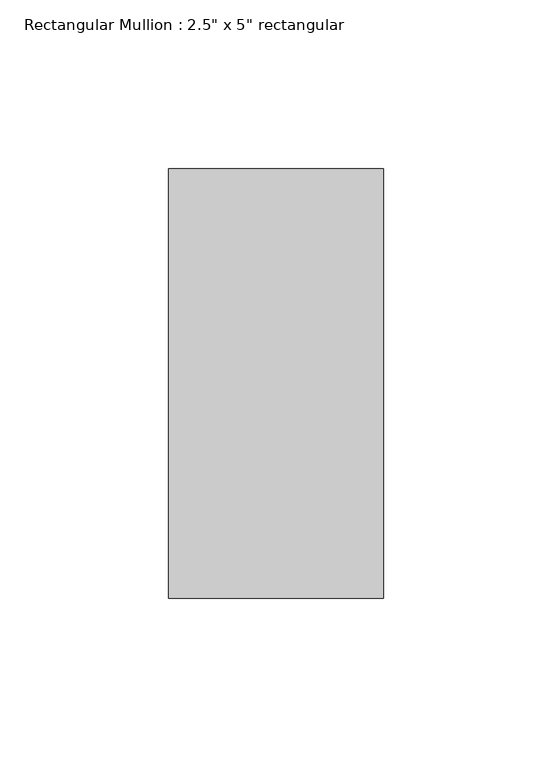
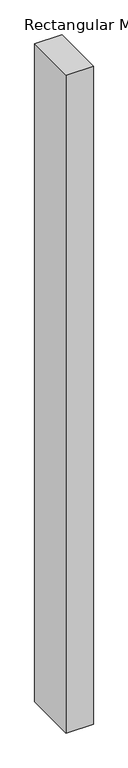
"""IFC4 building model written with IfcOpenShell, lengths in millimetres: member geometry."""

from ifc_helpers import new_model, si_unit, frame, origin, place, context, project, spatial, polyline, outline, extrude, source, transform, mapped, element, save


def member_bef6d027(model_context):
    return source(origin(), model_context, "Body", "SweptSolid", [
        extrude(outline(polyline([(31.75, 63.5), (31.75, -63.5), (-31.75, -63.5), (-31.75, 63.5), (31.75, 63.5)])), frame((0.0, 0.0, -1623.9353791), z_axis=(0.0, 0.0, 1.0), x_axis=(1.0, 0.0, 0.0)), (0.0, 0.0, 1.0), 1623.9353791),
    ])


if __name__ == "__main__":
    model = new_model("IFC4")
    model_context = context("Model", 3, world=origin())
    ifc_project = project(units=[si_unit("LENGTHUNIT", "METRE", prefix="MILLI")], contexts=[model_context])
    site = spatial("IfcSite", under=ifc_project)
    building = spatial("IfcBuilding", under=site)
    placement = place(None, origin())
    member_shape = member_bef6d027(model_context)
    element("IfcMember", 1, ObjectType="Rectangular Mullion : 2.5\" x 5\" rectangular", at=placement, inside=building, context=model_context, shape_type="MappedRepresentation", body=[
        mapped(member_shape, transform((0.0, 0.0, 0.0), x_axis=(1.0, 0.0, 0.0), y_axis=(0.0, 1.0, 0.0), z_axis=(0.0, 0.0, 1.0))),
    ])
    save(model, "model.ifc")

# Revit data of these elements
# Type "Rectangular Mullion : 2.5\" x 5\" rectangular"
#   built-in parameter 1007304 = 0.416667 (stored number, unit not read)
#   built-in parameter 1007301 = 0.104167 (stored number, unit not read)
#   built-in parameter 1007300 = 0.104167 (stored number, unit not read)
# Element 1 (IfcMember, "Rectangular Mullion : 2.5\" x 5\" rectangular")
#   Materials on its faces: "Aluminum"
# Materials
#   "Aluminum": class "Metal", colour RGB 247 247 247, transparency 0, Description = "Aluminum 6061", Cost = 0
